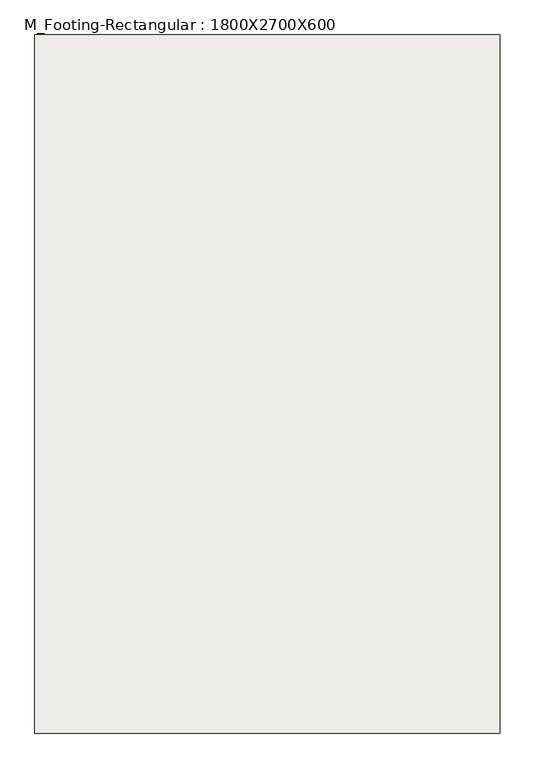
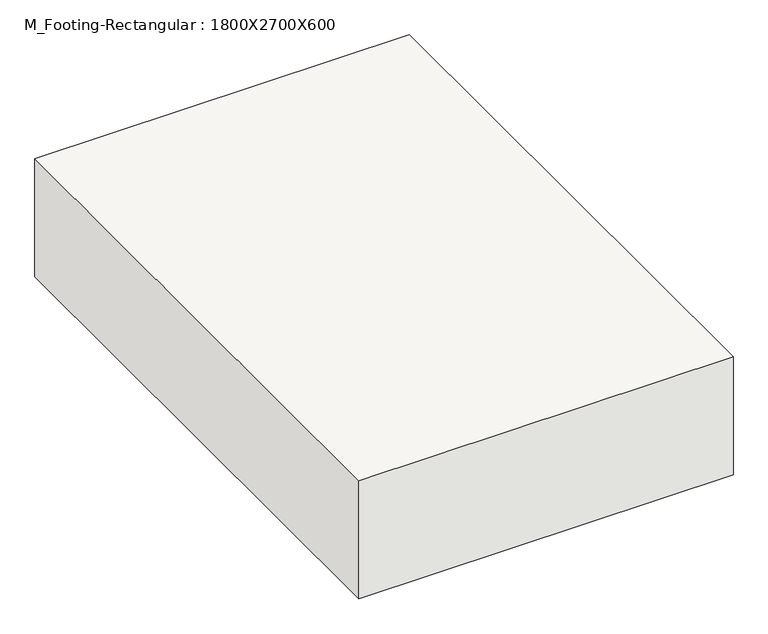
"""IFC4 building model written with IfcOpenShell, lengths in millimetres: slab geometry, M_Footing-Rectangular : 1800X2700X600."""

from ifc_helpers import new_model, si_unit, frame, origin, place, context, project, spatial, polyline, outline, extrude, source, transform, mapped, element, save


def m_footing_rectangular_1800x2700x600_14f11077(model_context):
    return source(origin(), model_context, "Body", "SweptSolid", [
        extrude(outline(polyline([(900.0, 1350.0), (900.0, -1350.0), (-900.0, -1350.0), (-900.0, 1350.0), (900.0, 1350.0)])), frame((0.0, 0.0, -600.0), z_axis=(0.0, 0.0, 1.0), x_axis=(1.0, 0.0, 0.0)), (0.0, 0.0, 1.0), 600.0),
    ])


if __name__ == "__main__":
    model = new_model("IFC4")
    model_context = context("Model", 3, world=origin())
    ifc_project = project(units=[si_unit("LENGTHUNIT", "METRE", prefix="MILLI")], contexts=[model_context])
    site = spatial("IfcSite", under=ifc_project)
    building = spatial("IfcBuilding", under=site)
    placement = place(None, origin())
    m_footing_rectangular_1800x2700x600_shape = m_footing_rectangular_1800x2700x600_14f11077(model_context)
    element("IfcSlab", 1, ObjectType="M_Footing-Rectangular : 1800X2700X600", at=placement, inside=building, context=model_context, shape_type="MappedRepresentation", body=[
        mapped(m_footing_rectangular_1800x2700x600_shape, transform((0.0, 0.0, 0.0), x_axis=(1.0, 0.0, 0.0), y_axis=(0.0, 1.0, 0.0), z_axis=(0.0, 0.0, 1.0))),
    ])
    save(model, "model.ifc")

# Revit data of these elements
# Type "M_Footing-Rectangular : 1800X2700X600"
#   Width = 1800 mm
#   Length = 2700 mm
#   Foundation Thickness = 600 mm
#   Structural Material [instance default] = Concrete, Cast-in-Place gray
#   Assembly Code = ""
# Element 1 (IfcSlab, "M_Footing-Rectangular : 1800X2700X600")
#   Structural Material = Concrete, Cast In Situ
#   Materials on its faces: "Concrete, Cast In Situ"
# Materials
#   "Concrete, Cast-in-Place gray": class "Concrete", colour RGB 192 192 192, transparency 0, Description = "Cast-in-place concrete", Cost = 0
#   "Concrete, Cast In Situ": class "Concrete", colour RGB 192 192 192, transparency 0, Description = "physical material", Cost = 0
